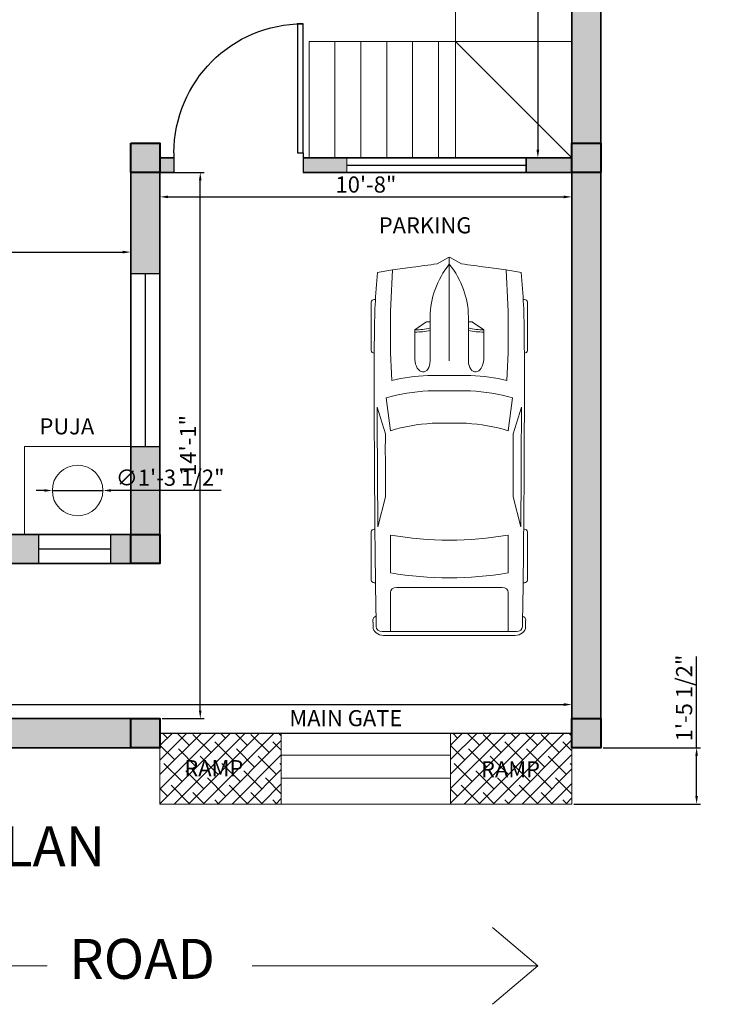
# Model space of a CAD drawing. Units: inches. Extents: x 1674 to 2231, y 1328 to 1959.
# Tile 2 of 6: x 1952 to 2166, y 1359 to 1664. Entities that reach past the tile are written whole.
import ezdxf

# ---------------------------------------------------------------- set-up
doc = ezdxf.new("R2010")
doc.units = ezdxf.units.IN
doc.linetypes.add('ACAD_ISO02W100', pattern=[15, 12, -3])
for name, color, linetype, lineweight in [('A-ANNO-DIMS', 113, 'Continuous', 18), ('A-ANNO-SYMB', 113, 'Continuous', 18), ('A-ANNO-TEXT', 113, 'Continuous', 18), ('A-AREA-IDEN', 113, 'Continuous', 18), ('A-COLS-PATT', 10, 'Continuous', 13), ('A-FLOR-CASE', 211, 'Continuous', 18), ('A-FLOR-STRS', 7, 'Continuous', 18), ('A-GLAZ-HIDN', 181, 'ACAD_ISO02W100', 18), ('A-SITE-GATE', 7, 'Continuous', 25), ('A-SITE-PATT', 8, 'Continuous', 13), ('A-SITE-PVMT', 7, 'Continuous', 18), ('A-SITE-VEHI', 211, 'Continuous', 13), ('A-WALL-PATT', 140, 'Continuous', 13), ('COLUMN', 10, 'Continuous', 40), ('DOOR', 54, 'Continuous', 25), ('WALL', 7, 'Continuous', 35), ('WN', 181, 'Continuous', 25)]:
    doc.layers.add(name, color=color, linetype=linetype, lineweight=lineweight)
doc.styles.get("Standard").update_dxf_attribs({"font": 'arial.ttf'})
doc.dimstyles.new('ISO-25', dxfattribs={"dimtxt": 5, "dimasz": 2.5, "dimexe": 1.25, "dimexo": 0.625, "dimtad": 1, "dimdec": 0, "dimlunit": 4, "dimtxsty": 'Standard', "dimcen": 2.5, "dimadec": 0, "dimazin": 0, "dimtfac": 1, "dimtdec": 0, "dimtmove": 0, "dimatfit": 3, "dimfxl": 1, "dimarcsym": 0})

# ---------------------------------------------------------------- blocks, each defined once
blk = doc.blocks.new('*U6')
for p, q in [((21.1, 37.41), (21.1, 36.83)), ((46.55, 38.89), (22.35, 38.89)), ((47.8, 37.39), (47.8, 37.41)), ((87.99, 31.87), (74.76, 35.92)), ((134.31, 35.6), (119.29, 31.78)), ((135.45, 37.07), (135.45, 37.41)), ((136.7, 38.89), (160.9, 38.89)), ((162.15, 37.41), (162.15, 36.77)), ((70.03, 31.54), (86.41, 29.35)), ((186.47, -33.5), (186.47, 33.5)), ((188.4, -32.76), (188.4, 32.76)), ((138.42, 29.35), (157.25, 29.35)), ((164.52, 26.39), (164.52, -26.39)), ((186.47, 29.35), (167.01, 29.35)), ((32.27, 11.63), (36.13, 17.17)), ((36.13, 17.17), (50.94, 17.17)), ((32.12, 9.51), (32.12, 11.15)), ((58.92, -10.77), (58.92, 10.77)), ((66.55, -10.53), (66.55, 10.53)), ((186.47, -10.53), (186.47, 10.53)), ((3.27, 6.13), (0.1, 0.41)), ((29.77, 9.51), (51.68, 9.51)), ((82.74, 8.5), (82.74, -8.5)), ((0, 0), (51.68, 0)), ((0.1, -0.41), (3.27, -6.13)), ((29.77, -9.51), (51.68, -9.51)), ((32.12, -9.51), (32.12, -11.15)), ((32.27, -11.63), (36.13, -17.17)), ((36.13, -17.17), (50.94, -17.17)), ((86.41, -29.35), (70.03, -31.54)), ((157.25, -29.35), (138.42, -29.35)), ((167.01, -29.35), (186.47, -29.35)), ((87.99, -31.87), (74.76, -35.92)), ((134.31, -35.6), (119.29, -31.78)), ((21.1, -37.41), (21.1, -36.83)), ((46.55, -38.89), (22.35, -38.89)), ((47.8, -37.39), (47.8, -37.41)), ((135.45, -37.07), (135.45, -37.41)), ((136.7, -38.89), (160.9, -38.89)), ((162.15, -37.41), (162.15, -36.77))]:
    blk.add_line(p, q)
for centre, major_axis, ratio, start_param, end_param in [((266.03, -27.52), (0, 313.31), 0.842304, 1.367076, 1.39176), ((41.19, -490.86), (0, 528.23), 0.842304, 0.00281, 0.075598), ((22.35, 37.41), (0, -1.48), 0.842304, 3.141593, 4.712389), ((64.48, -10555.62), (0, 10593.03), 0.842304, -0.013397, 0.002797), ((46.55, 37.41), (0, 1.48), 0.842304, -1.570796, 0), ((64.48, -10555.62), (0, -10591.55), 0.842304, 3.133765, 3.140441), ((136.7, 37.41), (0, -1.48), 0.842304, 3.141593, 4.712389), ((160.9, 37.41), (0, 1.48), 0.842304, -1.570796, 0), ((180.63, 35.84), (0, 2.22), 0.842304, -0.013017, 1.249894), ((64.48, -10556.36), (0, 10595.31), 0.842304, -0.013397, -0.013017), ((183.98, 33.5), (0, -2.96), 0.842304, 1.570796, 3.128196), ((183.98, 32.76), (0, -5.25), 0.842304, 1.570796, 3.128196), ((37.47, -593.96), (0, -623.33), 0.842304, 3.096046, 3.200911), ((135.29, 5.39), (0, 81.77), 0.842304, 1.245306, 1.50788), ((95.79, -3666.35), (0, -3698.24), 0.842304, 3.134049, 3.144098), ((259.18, -27.52), (0, -305.3), 0.842304, 4.528606, 4.561838), ((134.4, 5.39), (0, -89.78), 0.842304, 4.449482, 4.652344), ((149.6, 2.8), (0, -79.58), 0.842304, 4.372215, 4.640744), ((17.08, 0), (0, 147.02), 0.842304, 4.511394, 4.913384), ((35.91, 0), (0, 147.02), 0.842304, 4.511394, 4.913384), ((167.01, 26.39), (0, 2.96), 0.842304, 0, 1.570796), ((-204.49, 52.4), (0, -250.96), 0.842304, 1.385369, 1.434372), ((13.04, 17.01), (0, 27.42), 0.842304, 4.435146, 4.718221), ((14.2, 17.01), (0, 27.42), 0.842304, 4.435146, 4.718221), ((50.79, 13.34), (6.34, -0.36), 0.603834, -1.395552, 1.581315), ((32.75, 11.15), (0, 0.74), 0.842304, 0.879714, 1.570796), ((29.77, -46.66), (0, 56.17), 0.842304, 0, 0.590319), ((0.62, 0), (0, -0.74), 0.842304, 4.131459, 5.293319), ((29.77, 46.66), (0, 56.17), 0.842304, 2.551274, 3.141593), ((-204.49, -52.4), (0, 250.96), 0.842304, -1.434372, -1.385369), ((13.04, -17.01), (0, -27.42), 0.842304, 1.564964, 1.848039), ((14.2, -17.01), (0, -27.42), 0.842304, 1.564964, 1.848039), ((149.6, -2.8), (0, -79.58), 0.842304, -1.499151, -1.230623), ((32.75, -11.15), (0, -0.74), 0.842304, 4.712389, 5.403472), ((134.4, -5.39), (0, -89.78), 0.842304, -1.510751, -1.307889), ((135.29, -5.39), (0, -81.77), 0.842304, -1.50788, -1.245306), ((259.18, 27.52), (0, 305.3), 0.842304, 1.721348, 1.754579), ((266.03, 27.52), (0, 313.31), 0.842304, 1.749832, 1.774517), ((37.47, 593.96), (0, -623.33), 0.842304, -0.059319, 0.045547), ((167.01, -26.39), (0, -2.96), 0.842304, 4.712389, 6.283185), ((95.79, 3666.35), (0, -3698.24), 0.842304, -0.002505, 0.007544), ((183.98, -33.5), (0, 2.96), 0.842304, 3.15499, 4.712389), ((183.98, -32.76), (0, -5.25), 0.842304, 0.013397, 1.570796), ((41.19, 490.86), (0, -528.23), 0.842304, -0.075598, -0.00281), ((22.35, -37.41), (0, 1.48), 0.842304, 1.570796, 3.141593), ((64.48, 10555.62), (0, 10593.03), 0.842304, 3.138796, 3.15499), ((46.55, -37.41), (0, -1.48), 0.842304, 0, 1.570796), ((64.48, 10555.62), (0, -10591.55), 0.842304, 0.001152, 0.007828), ((136.7, -37.41), (0, -1.48), 0.842304, -1.570796, 0), ((160.9, -37.41), (0, 1.48), 0.842304, 3.141593, 4.712389), ((180.63, -35.84), (0, -2.22), 0.842304, -1.249894, 0.013017), ((64.48, 10556.36), (0, 10595.31), 0.842304, 3.15461, 3.15499)]:
    blk.add_ellipse(centre, major_axis=major_axis, ratio=ratio, start_param=start_param, end_param=end_param)
at = {"extrusion": (0, 0, -1)}
blk.add_ellipse((50.79, -13.34), major_axis=(6.34, 0.36), ratio=0.603834, start_param=-1.395552, end_param=1.581315, dxfattribs=at)
blk = doc.blocks.new('*U2')
for p, q in [((0, 0), (0, -6)), ((40, 0), (40, -6))]:
    blk.add_line(p, q)
blk.add_lwpolyline([(0, 0), (0, 40), (1.75, 40), (1.75, 0)], close=True)
blk.add_arc((0, 0), 40, 0, 90)
blk = doc.blocks.new('*D21')
at = {"layer": 'A-ANNO-DIMS', "color": 0, "lineweight": -2, "transparency": 16777216}
for p, q in [((2122.65, 1748.86), (2111.49, 1748.86)), ((2112.74, 1746.36), (2112.74, 1623.36)), ((2122.65, 1620.86), (2111.49, 1620.86))]:
    blk.add_line(p, q, dxfattribs=at)
at = {"layer": 'A-ANNO-DIMS', "color": 0, "lineweight": 100, "transparency": 16777216}
for points in [[(2112.32, 1746.36), (2113.15, 1746.36), (2112.74, 1748.86)], [(2112.32, 1623.36), (2113.15, 1623.36), (2112.74, 1620.86)]]:
    blk.add_solid(points, dxfattribs=at)
at = {"layer": 'Defpoints', "color": 0, "lineweight": 100, "transparency": 16777216}
for p in [(2123.27, 1748.86), (2112.74, 1620.86), (2123.27, 1620.86)]:
    blk.add_point(p, dxfattribs=at)
at = {"layer": 'A-ANNO-DIMS', "color": 0, "transparency": 16777216, "insert": (2109.56, 1684.86), "char_height": 5, "attachment_point": 5, "rotation": 90}
blk.add_mtext('10\'-8"', dxfattribs=at)
blk = doc.blocks.new('*D29')
at = {"layer": 'A-ANNO-DIMS', "color": 0, "lineweight": -2, "transparency": 16777216}
for p, q in [((1745.27, 1447.98), (1745.27, 1452.95)), ((1747.77, 1451.7), (2120.77, 1451.7)), ((2123.27, 1447.98), (2123.27, 1452.95))]:
    blk.add_line(p, q, dxfattribs=at)
at = {"layer": 'A-ANNO-DIMS', "color": 0, "lineweight": 100, "transparency": 16777216}
for points in [[(1747.77, 1452.12), (1747.77, 1451.28), (1745.27, 1451.7)], [(2120.77, 1452.12), (2120.77, 1451.28), (2123.27, 1451.7)]]:
    blk.add_solid(points, dxfattribs=at)
at = {"layer": 'Defpoints', "color": 0, "lineweight": 100, "transparency": 16777216}
for p in [(2123.27, 1451.7), (1745.27, 1447.36), (2123.27, 1447.36)]:
    blk.add_point(p, dxfattribs=at)
at = {"layer": 'A-ANNO-DIMS', "color": 0, "transparency": 16777216, "insert": (1934.27, 1454.88), "char_height": 5, "attachment_point": 5}
blk.add_mtext('31\'-6"', dxfattribs=at)
blk = doc.blocks.new('*D30')
at = {"layer": 'A-ANNO-DIMS', "color": 0, "lineweight": -2, "transparency": 16777216}
for p, q in [((1869.77, 1504.98), (1869.77, 1592.95)), ((1872.27, 1591.7), (1984.27, 1591.7)), ((1986.77, 1504.98), (1986.77, 1592.95))]:
    blk.add_line(p, q, dxfattribs=at)
at = {"layer": 'A-ANNO-DIMS', "color": 0, "lineweight": 100, "transparency": 16777216}
for points in [[(1872.27, 1592.11), (1872.27, 1591.28), (1869.77, 1591.7)], [(1984.27, 1592.11), (1984.27, 1591.28), (1986.77, 1591.7)]]:
    blk.add_solid(points, dxfattribs=at)
at = {"layer": 'Defpoints', "color": 0, "lineweight": 100, "transparency": 16777216}
for p in [(1986.77, 1591.7), (1869.77, 1504.36), (1986.77, 1504.36)]:
    blk.add_point(p, dxfattribs=at)
at = {"layer": 'A-ANNO-DIMS', "color": 0, "transparency": 16777216, "insert": (1928.27, 1594.88), "char_height": 5, "attachment_point": 5}
blk.add_mtext('9\'-9"', dxfattribs=at)
blk = doc.blocks.new('*D31')
at = {"layer": 'A-ANNO-DIMS', "color": 0, "lineweight": -2, "transparency": 16777216}
for p, q in [((1996.4, 1616.36), (2009.49, 1616.36)), ((2008.24, 1449.86), (2008.24, 1613.86)), ((1996.4, 1447.36), (2009.49, 1447.36))]:
    blk.add_line(p, q, dxfattribs=at)
at = {"layer": 'A-ANNO-DIMS', "color": 0, "lineweight": 100, "transparency": 16777216}
for points in [[(2007.82, 1613.86), (2008.65, 1613.86), (2008.24, 1616.36)], [(2007.82, 1449.86), (2008.65, 1449.86), (2008.24, 1447.36)]]:
    blk.add_solid(points, dxfattribs=at)
at = {"layer": 'Defpoints', "color": 0, "lineweight": 100, "transparency": 16777216}
for p in [(1995.77, 1616.36), (2008.24, 1616.36), (1995.77, 1447.36)]:
    blk.add_point(p, dxfattribs=at)
at = {"layer": 'A-ANNO-DIMS', "color": 0, "transparency": 16777216, "insert": (2005.1, 1531.86), "char_height": 5, "attachment_point": 5, "rotation": 90}
blk.add_mtext('14\'-1"', dxfattribs=at)
blk = doc.blocks.new('*D32')
at = {"layer": 'A-ANNO-DIMS', "color": 0, "lineweight": -2, "transparency": 16777216}
for p, q in [((1995.77, 1615.73), (1995.77, 1607.53)), ((2123.27, 1615.73), (2123.27, 1607.53)), ((1998.27, 1608.78), (2120.77, 1608.78))]:
    blk.add_line(p, q, dxfattribs=at)
at = {"layer": 'A-ANNO-DIMS', "color": 0, "lineweight": 100, "transparency": 16777216}
for points in [[(1998.27, 1609.19), (1998.27, 1608.36), (1995.77, 1608.78)], [(2120.77, 1609.19), (2120.77, 1608.36), (2123.27, 1608.78)]]:
    blk.add_solid(points, dxfattribs=at)
at = {"layer": 'Defpoints', "color": 0, "lineweight": 100, "transparency": 16777216}
for p in [(1995.77, 1616.36), (2123.27, 1616.36), (2123.27, 1608.78)]:
    blk.add_point(p, dxfattribs=at)
at = {"layer": 'A-ANNO-DIMS', "color": 0, "transparency": 16777216, "insert": (2059.52, 1611.96), "char_height": 5, "attachment_point": 5}
blk.add_mtext('10\'-8"', dxfattribs=at)
blk = doc.blocks.new('ARROW-ROAD-DIRECTION')
for p, q in [((0, 11.86), (14.05, 23.72)), ((88.42, 11.86), (0, 11.86)), ((4.6, 11.86), (0, 11.86)), ((0, 11.86), (14.05, 0))]:
    blk.add_line(p, q)
blk = doc.blocks.new('*D50')
at = {"layer": 'A-ANNO-DIMS', "color": 0, "lineweight": -2, "transparency": 16777216}
for p, q in [((2161.87, 1438.36), (2161.87, 1466.58)), ((2132.9, 1438.36), (2163.12, 1438.36)), ((2161.87, 1423.43), (2161.87, 1435.86)), ((2123.9, 1420.93), (2163.12, 1420.93))]:
    blk.add_line(p, q, dxfattribs=at)
at = {"layer": 'A-ANNO-DIMS', "color": 0, "lineweight": 100, "transparency": 16777216}
for points in [[(2161.45, 1435.86), (2162.29, 1435.86), (2161.87, 1438.36)], [(2161.45, 1423.43), (2162.29, 1423.43), (2161.87, 1420.93)]]:
    blk.add_solid(points, dxfattribs=at)
at = {"layer": 'Defpoints', "color": 0, "lineweight": 100, "transparency": 16777216}
for p in [(2132.27, 1438.36), (2161.87, 1438.36), (2123.27, 1420.93)]:
    blk.add_point(p, dxfattribs=at)
at = {"layer": 'A-ANNO-DIMS', "color": 0, "transparency": 16777216, "insert": (2158.66, 1453.72), "char_height": 5, "attachment_point": 5, "rotation": 90}
blk.add_mtext('1\'-5 1/2"', dxfattribs=at)
blk = doc.blocks.new('*D58')
at = {"layer": 'A-ANNO-DIMS', "color": 0, "lineweight": -2, "transparency": 16777216}
for p, q in [((1959.96, 1517.93), (1957.46, 1517.93)), ((1962.46, 1517.93), (1978.11, 1517.93)), ((2014.75, 1517.93), (1980.61, 1517.93))]:
    blk.add_line(p, q, dxfattribs=at)
at = {"layer": 'A-ANNO-DIMS', "color": 0, "lineweight": 100, "transparency": 16777216}
for points in [[(1959.96, 1518.35), (1959.96, 1517.52), (1962.46, 1517.93)], [(1980.61, 1518.35), (1980.61, 1517.52), (1978.11, 1517.93)]]:
    blk.add_solid(points, dxfattribs=at)
at = {"layer": 'Defpoints', "color": 0, "lineweight": 100, "transparency": 16777216}
for p in [(1962.46, 1517.93), (1978.11, 1517.93)]:
    blk.add_point(p, dxfattribs=at)
at = {"layer": 'A-ANNO-DIMS', "color": 0, "transparency": 16777216, "insert": (1998.93, 1521.25), "char_height": 5, "attachment_point": 5, "rotation": 0.0005}
blk.add_mtext('∅1\'-3 1/2"', dxfattribs=at)

msp = doc.modelspace()

# ---------------------------------------------------------------- hatches: boundary and pattern name
at = {"layer": 'A-COLS-PATT'}
h = msp.add_hatch(color=256, dxfattribs=at)
h.dxf.hatch_style = 1
h.paths.add_polyline_path([(1745.27, 1918.36), (1736.27, 1918.36), (1736.27, 1909.36), (1745.27, 1909.36)])
h.paths.add_polyline_path([(1886.27, 1918.36), (1877.27, 1918.36), (1877.27, 1909.36), (1886.27, 1909.36)])
h.paths.add_polyline_path([(1995.77, 1918.36), (1986.77, 1918.36), (1986.77, 1909.36), (1995.77, 1909.36)])
h.paths.add_polyline_path([(2132.27, 1918.36), (2123.27, 1918.36), (2123.27, 1909.36), (2132.27, 1909.36)])
h.paths.add_polyline_path([(1745.27, 1757.86), (1736.27, 1757.86), (1736.27, 1748.86), (1745.27, 1748.86)])
h.paths.add_polyline_path([(1886.27, 1757.86), (1877.27, 1757.86), (1877.27, 1748.86), (1886.27, 1748.86)])
h.paths.add_polyline_path([(2132.27, 1757.81), (2123.27, 1757.81), (2123.27, 1748.81), (2132.27, 1748.81)])
h.paths.add_polyline_path([(1995.77, 1757.86), (1986.77, 1757.86), (1986.77, 1748.86), (1995.77, 1748.86)])
h.paths.add_polyline_path([(2132.27, 1625.36), (2123.27, 1625.36), (2123.27, 1616.36), (2132.27, 1616.36)])
h.paths.add_polyline_path([(1995.77, 1625.36), (1986.77, 1625.36), (1986.77, 1616.36), (1995.77, 1616.36)])
h.paths.add_polyline_path([(1869.77, 1604.86), (1860.77, 1604.86), (1860.77, 1595.86), (1869.77, 1595.86)])
h.paths.add_polyline_path([(1745.27, 1609.36), (1736.27, 1609.36), (1736.27, 1600.36), (1745.27, 1600.36)])
h.paths.add_polyline_path([(1745.27, 1504.36), (1736.27, 1504.36), (1736.27, 1495.36), (1745.27, 1495.36)])
h.paths.add_polyline_path([(1870.95, 1504.36), (1861.95, 1504.36), (1861.95, 1495.36), (1870.95, 1495.36)])
h.paths.add_polyline_path([(1995.77, 1504.36), (1986.77, 1504.36), (1986.77, 1495.36), (1995.77, 1495.36)])
h.paths.add_polyline_path([(1995.77, 1447.36), (1986.77, 1447.36), (1986.77, 1438.36), (1995.77, 1438.36)])
h.paths.add_polyline_path([(2132.27, 1447.36), (2123.27, 1447.36), (2123.27, 1438.36), (2132.27, 1438.36)])
at = {"layer": 'A-SITE-PATT'}
h = msp.add_hatch(dxfattribs=at)
h.set_pattern_fill('ANSI38', color=256)
h.paths.add_polyline_path([(2033.3, 1442.86), (1995.77, 1442.86), (1995.77, 1420.93), (2033.3, 1420.93)])
h.paths.add_polyline_path([(2123.27, 1442.86), (2085.74, 1442.86), (2085.74, 1420.93), (2123.27, 1420.93)])
at = {"layer": 'A-WALL-PATT'}
h = msp.add_hatch(color=256, dxfattribs=at)
h.dxf.hatch_style = 1
h.paths.add_polyline_path([(2132.27, 1909.36), (2123.27, 1909.36), (2123.27, 1757.81), (2132.27, 1757.81)], flags=17)
h.paths.add_polyline_path([(2123.27, 1753.36), (2040.84, 1753.36), (2040.84, 1748.86), (2123.27, 1748.86)], flags=17)
h.paths.add_polyline_path([(1840.51, 1753.36), (1745.27, 1753.36), (1745.27, 1748.86), (1817.27, 1748.86), (1840.51, 1748.86)], flags=17)
h.paths.add_polyline_path([(1745.27, 1748.86), (1736.27, 1748.86), (1736.27, 1609.36), (1745.27, 1609.36), (1745.27, 1640.86)], flags=17)
h.paths.add_polyline_path([(1745.27, 1600.36), (1736.27, 1600.36), (1736.27, 1504.36), (1745.27, 1504.36)], flags=17)
h.paths.add_polyline_path([(1745.27, 1495.36), (1736.27, 1495.36), (1736.27, 1447.36), (1745.27, 1447.36)], flags=17)
h.paths.add_polyline_path([(1820.35, 1504.36), (1787.69, 1504.36), (1787.69, 1495.36), (1820.35, 1495.36)], flags=17)
h.paths.add_polyline_path([(1750.58, 1504.36), (1745.27, 1504.36), (1745.27, 1495.36), (1750.58, 1495.36)], flags=17)
h.paths.add_polyline_path([(1861.95, 1504.36), (1857.47, 1504.36), (1857.47, 1495.36), (1861.95, 1495.36)], flags=17)
h.paths.add_polyline_path([(1873.66, 1504.36), (1870.95, 1504.36), (1870.95, 1495.36), (1873.66, 1495.36)], flags=17)
h.paths.add_polyline_path([(1900.85, 1501.36), (1900.85, 1504.36), (1895.88, 1504.36), (1895.88, 1495.36), (1900.85, 1495.36)], flags=17)
h.paths.add_polyline_path([(1869.77, 1595.86), (1865.27, 1595.86), (1865.27, 1504.36), (1869.77, 1504.36)], flags=17)
h.paths.add_polyline_path([(1958.26, 1504.36), (1940.74, 1504.36, -0.01877), (1940.85, 1501.36), (1940.85, 1495.36), (1958.26, 1495.36)], flags=17)
h.paths.add_polyline_path([(1995.77, 1531.51), (1986.77, 1531.51), (1986.77, 1504.36), (1995.77, 1504.36)], flags=17)
h.paths.add_polyline_path([(1986.77, 1504.36), (1980.49, 1504.36), (1980.49, 1495.36), (1986.77, 1495.36)], flags=17)
h.paths.add_polyline_path([(1995.77, 1616.36), (1986.77, 1616.36), (1986.77, 1585.02), (1995.77, 1585.02)], flags=17)
h.paths.add_polyline_path([(2000.1, 1620.86), (1995.77, 1620.86), (1995.77, 1616.36), (2000.1, 1616.36)], flags=17)
h.paths.add_polyline_path([(2053.57, 1620.86), (2040.1, 1620.86), (2040.1, 1616.36), (2053.57, 1616.36)], flags=17)
h.paths.add_polyline_path([(2123.27, 1620.86), (2109.12, 1620.86), (2109.12, 1616.36), (2123.27, 1616.36)], flags=17)
h.paths.add_polyline_path([(2132.27, 1616.36), (2123.27, 1616.36), (2123.27, 1447.36), (2132.27, 1447.36)], flags=17)
h.paths.add_polyline_path([(1986.77, 1447.36), (1870.95, 1447.36), (1870.95, 1438.36), (1986.77, 1438.36)])
h.paths.add_polyline_path([(1861.95, 1447.36), (1745.27, 1447.36), (1745.27, 1438.36), (1861.95, 1438.36)])
h.paths.add_polyline_path([(2132.27, 1918.36), (1736.27, 1918.36), (1736.27, 1504.36), (1745.27, 1504.36), (1745.27, 1600.36), (1745.27, 1909.36), (2123.27, 1909.36), (2123.27, 1447.36), (2132.27, 1447.36)])
h = msp.add_hatch(color=256, dxfattribs=at)
h.dxf.hatch_style = 1
h.paths.add_polyline_path([(2132.27, 1616.36), (2123.27, 1616.36), (2123.27, 1447.36), (2132.27, 1447.36)])

# ---------------------------------------------------------------- linework, layer by layer
at = {"layer": 'A-FLOR-CASE'}
msp.add_lwpolyline([(1986.77, 1531.51), (1953.8, 1531.51), (1953.8, 1504.36), (1986.77, 1504.36)], close=True, dxfattribs=at)
msp.add_circle((1970.28, 1517.93), 7.83, dxfattribs=at)
at = {"layer": 'A-FLOR-STRS'}
for p, q in [((2087.27, 1656.86), (2087.27, 1712.86)), ((2041.94, 1620.86), (2041.94, 1656.86)), ((2041.94, 1656.86), (2087.27, 1656.86)), ((2049.94, 1620.86), (2049.94, 1656.86)), ((2057.94, 1620.86), (2057.94, 1656.86)), ((2065.94, 1620.86), (2065.94, 1656.86)), ((2073.94, 1620.86), (2073.94, 1656.86)), ((2081.94, 1620.86), (2081.94, 1656.86)), ((2087.27, 1656.86), (2087.27, 1620.86)), ((2087.27, 1656.86), (2123.27, 1656.86)), ((2087.27, 1656.86), (2123.27, 1620.86))]:
    msp.add_line(p, q, dxfattribs=at)
at = {"layer": 'A-GLAZ-HIDN'}
msp.add_line((2053.57, 1620.86), (2053.57, 1616.36), dxfattribs=at)
msp.add_lwpolyline([(2053.57, 1616.36), (2109.12, 1616.36), (2109.12, 1620.86), (2053.57, 1620.86)], close=True, dxfattribs=at)
at = {"layer": 'A-SITE-GATE'}
msp.add_line((1995.77, 1442.86), (2123.27, 1442.86), dxfattribs=at)
at = {"layer": 'A-SITE-PVMT'}
for p, q in [((2033.3, 1436.04), (2085.74, 1436.04)), ((2033.3, 1428.91), (2085.74, 1428.91)), ((2033.3, 1420.93), (2085.74, 1420.93))]:
    msp.add_line(p, q, dxfattribs=at)
for points in [[(1995.77, 1442.86), (2033.3, 1442.86), (2033.3, 1420.93), (1995.77, 1420.93)], [(2085.74, 1442.86), (2123.27, 1442.86), (2123.27, 1420.93), (2085.74, 1420.93)]]:
    msp.add_lwpolyline(points, close=True, dxfattribs=at)
at = {"layer": 'COLUMN'}
for points in [[(1986.77, 1625.36), (1995.77, 1625.36), (1995.77, 1616.36), (1986.77, 1616.36)], [(2123.27, 1625.36), (2132.27, 1625.36), (2132.27, 1616.36), (2123.27, 1616.36)], [(1986.77, 1504.36), (1995.77, 1504.36), (1995.77, 1495.36), (1986.77, 1495.36)], [(1986.77, 1447.36), (1995.77, 1447.36), (1995.77, 1438.36), (1986.77, 1438.36)], [(2123.27, 1447.36), (2132.27, 1447.36), (2132.27, 1438.36), (2123.27, 1438.36)]]:
    msp.add_lwpolyline(points, close=True, dxfattribs=at)
at = {"layer": 'WALL'}
for p, q in [((2132.27, 1918.36), (2132.27, 1438.36)), ((1986.77, 1620.86), (1986.77, 1504.36)), ((1995.77, 1620.86), (1995.77, 1495.36)), ((2000.1, 1620.86), (1995.77, 1620.86)), ((2123.27, 1620.86), (2040.1, 1620.86)), ((2000.1, 1616.36), (1995.77, 1616.36)), ((2132.27, 1616.36), (2040.1, 1616.36)), ((2132.27, 1438.36), (2132.27, 1616.36)), ((1940.74, 1504.36), (1986.77, 1504.36)), ((1940.85, 1495.36), (1995.77, 1495.36)), ((1995.77, 1438.36), (1736.27, 1438.36)), ((2132.27, 1438.36), (2123.27, 1438.36))]:
    msp.add_line(p, q, dxfattribs=at)
for points in [[(1995.77, 1438.36), (1736.27, 1438.36), (1736.27, 1918.36), (2132.27, 1918.36), (2132.27, 1438.36), (2123.27, 1438.36)], [(1995.77, 1447.36), (1745.27, 1447.36), (1745.27, 1909.36), (2123.27, 1909.36), (2123.27, 1447.36)], [(2040.1, 1616.36), (2109.12, 1616.36), (2109.12, 1620.86), (2040.1, 1620.86)]]:
    msp.add_lwpolyline(points, dxfattribs=at)
at = {"layer": 'WN'}
for p, q in [((2053.57, 1618.61), (2109.12, 1618.61)), ((1991.27, 1531.51), (1991.27, 1585.02)), ((1958.26, 1499.86), (1980.49, 1499.86))]:
    msp.add_line(p, q, dxfattribs=at)
for points in [[(1995.77, 1585.02), (1986.77, 1585.02), (1986.77, 1531.51), (1995.77, 1531.51)], [(1958.26, 1504.36), (1980.49, 1504.36), (1980.49, 1495.36), (1958.26, 1495.36)]]:
    msp.add_lwpolyline(points, close=True, dxfattribs=at)

# ---------------------------------------------------------------- block references
at = {"layer": 'A-ANNO-SYMB'}
msp.add_blockref('ARROW-ROAD-DIRECTION', (1872.46, 1358.96), dxfattribs=at)
at = {"layer": 'A-ANNO-SYMB', "rotation": 180}
msp.add_blockref('ARROW-ROAD-DIRECTION', (2112.76, 1382.68), dxfattribs=at)
at = {"layer": 'A-SITE-VEHI', "xscale": 0.6211139060494296, "yscale": 0.6211139060494296, "zscale": 0.6211139060494296, "rotation": 270}
msp.add_blockref('*U6', (2085.33, 1590.11), dxfattribs=at)
at = {"layer": 'DOOR', "xscale": -1}
msp.add_blockref('*U2', (2040.1, 1622.36), dxfattribs=at)

# ---------------------------------------------------------------- texts
at = {"layer": 'A-ANNO-TEXT', "attachment_point": 1}
for s, width, gutter_width, insert, char_height in [('MAIN GATE', 89.7127, 24.87, (2035.85, 1449.98), 4.973), ('RAMP', 89.7127, 24.87, (2003.31, 1434.51), 4.973), ('RAMP', 89.7127, 24.87, (2095.15, 1434.14), 4.973), ('GROUND FLOOR PLAN', 223.3864, 61.92, (1803.67, 1414.03), 12.3835), ('ROAD', 223.3864, 61.92, (1967.63, 1379.21), 12.383)]:
    msp.add_mtext_dynamic_manual_height_columns(s, width=width, gutter_width=gutter_width, heights=[0], dxfattribs=dict(at, insert=insert, char_height=char_height))
at = {"layer": 'A-AREA-IDEN', "char_height": 4.973, "attachment_point": 1}
for s, insert in [('PARKING', (2063.5, 1602.47)), ('PUJA', (1958.48, 1540.27))]:
    msp.add_mtext_dynamic_manual_height_columns(s, width=89.7127, gutter_width=24.87, heights=[0], dxfattribs=dict(at, insert=insert))

# ---------------------------------------------------------------- dimensions: what is measured, and where the dimension line sits
at = {"layer": 'A-ANNO-DIMS'}
for base, p1, p2, override, picture, middle in [((2112.74, 1620.86), (2123.27, 1748.86), (2123.27, 1620.86), {"dimclrd": 0, "dimclre": 0, "dimclrt": 0}, '*D21', (2109.56, 1684.86)), ((2008.24, 1616.36), (1995.77, 1447.36), (1995.77, 1616.36), {"dimclrd": 0, "dimclre": 0, "dimclrt": 0}, '*D31', (2005.1, 1531.86)), ((2161.87, 1438.36), (2123.27, 1420.93), (2132.27, 1438.36), {"dimdec": 1, "dimlfac": 1, "dimrnd": 0, "dimzin": 1, "dimdsep": 46, "dimlunit": 4, "dimfrac": 2}, '*D50', (2158.66, 1453.72))]:
    dim = msp.add_linear_dim(base=base, p1=p1, p2=p2, angle=90, dimstyle='ISO-25', override=override, dxfattribs=at)
    dim.commit()
    dim.dimension.update_dxf_attribs({"geometry": picture, "text_midpoint": middle})
for base, p1, p2, picture, middle in [((2123.27109151, 1608.77774913), (1995.77109151, 1616.35548105), (2123.27109151, 1616.35548105), '*D32', (2059.52109151, 1611.95561407)), ((1986.77, 1591.7), (1869.77, 1504.36), (1986.77, 1504.36), '*D30', (1928.27, 1594.88)), ((2123.27, 1451.7), (1745.27, 1447.36), (2123.27, 1447.36), '*D29', (1934.27, 1454.88))]:
    dim = msp.add_linear_dim(base=base, p1=p1, p2=p2, dimstyle='ISO-25', override={"dimclrd": 0, "dimclre": 0, "dimclrt": 0}, dxfattribs=at)
    dim.commit()
    dim.dimension.update_dxf_attribs({"geometry": picture, "text_midpoint": middle})
dim = msp.add_diameter_dim_2p(p1=(1962.4555, 1517.9339), p2=(1978.1135, 1517.934), dimstyle='ISO-25', override={"dimdec": 1, "dimlfac": 1, "dimrnd": 0, "dimzin": 1, "dimdsep": 46, "dimlunit": 4, "dimfrac": 2}, dxfattribs=at)
dim.commit()
dim.dimension.update_dxf_attribs({"geometry": '*D58', "text_midpoint": (1998.9295, 1517.9342)})

doc.saveas('drawing.dxf')
